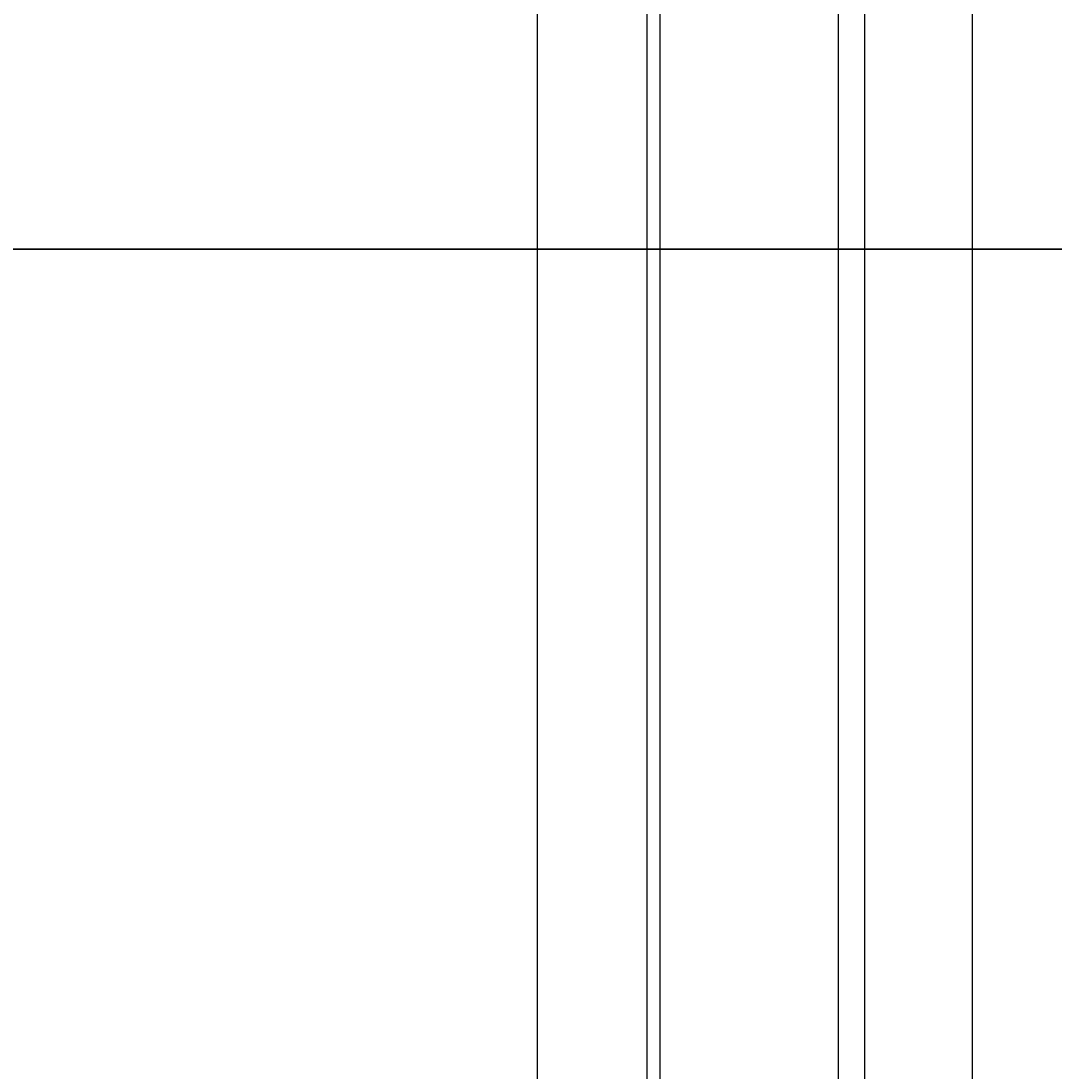
# Model space of a CAD drawing. Units: inches. Extents: x -6 to 289, y -8 to 323.
# Tile 81 of 107: x 150 to 173, y 229 to 252. Entities that reach past the tile are written whole.
import ezdxf

# ---------------------------------------------------------------- set-up
doc = ezdxf.new("R2010")
doc.units = ezdxf.units.IN
doc.header["$MEASUREMENT"] = 0
doc.layers.add('A-ANNO-DIMS', color=2, linetype='Continuous', lineweight=18)
doc.layers.add('A-ELEV', color=7, linetype='Continuous', lineweight=35)
doc.styles.get("Standard").update_dxf_attribs({"font": 'arial.ttf'})
doc.dimstyles.get("Standard").update_dxf_attribs({"dimtxt": 0.18, "dimasz": 0.18, "dimexe": 0.18, "dimexo": 0.0625, "dimgap": 0.09, "dimtad": 0, "dimtih": 1, "dimtoh": 1, "dimdec": 4, "dimzin": 0, "dimdsep": 46, "dimtxsty": 'Standard', "dimcen": 0.09, "dimadec": 0, "dimazin": 0, "dimtfac": 1, "dimtdec": 4, "dimtofl": 0, "dimtmove": 0, "dimatfit": 3, "dimfxl": 1, "dimtolj": 1, "dimtzin": 0, "dimarcsym": 0})

# ---------------------------------------------------------------- blocks, each defined once
blk = doc.blocks.new('*D11')
at = {"layer": 'A-ANNO-DIMS', "color": 0, "lineweight": -2, "transparency": 16777216}
for p, q in [((126.883, 226.717), (126.883, 322.969)), ((168.883, 226.717), (168.883, 322.969)), ((127.063, 322.789), (147.662, 322.789)), ((168.703, 322.789), (148.105, 322.789))]:
    blk.add_line(p, q, dxfattribs=at)
at = {"layer": 'A-ANNO-DIMS', "color": 0, "transparency": 16777216}
for points in [[(127.063, 322.819), (127.063, 322.759), (126.883, 322.789)], [(168.703, 322.819), (168.703, 322.759), (168.883, 322.789)]]:
    blk.add_solid(points, dxfattribs=at)
at = {"layer": 'Defpoints', "color": 0, "transparency": 16777216}
for p in [(168.883, 322.789), (126.883, 226.654), (168.883, 226.654)]:
    blk.add_point(p, dxfattribs=at)
at = {"layer": 'A-ANNO-DIMS', "color": 0, "transparency": 16777216, "insert": (147.883, 322.789), "char_height": 0.18, "attachment_point": 5}
blk.add_mtext('\\A1;42', dxfattribs=at)
blk = doc.blocks.new('*D12')
at = {"layer": 'A-ANNO-DIMS', "color": 0, "lineweight": -2, "transparency": 16777216}
for p, q in [((168.883, 226.717), (168.883, 322.969)), ((188.292, 226.951), (188.292, 322.969)), ((169.063, 322.789), (178.22, 322.789)), ((188.112, 322.789), (178.955, 322.789))]:
    blk.add_line(p, q, dxfattribs=at)
at = {"layer": 'A-ANNO-DIMS', "color": 0, "transparency": 16777216}
for points in [[(169.063, 322.819), (169.063, 322.759), (168.883, 322.789)], [(188.112, 322.819), (188.112, 322.759), (188.292, 322.789)]]:
    blk.add_solid(points, dxfattribs=at)
at = {"layer": 'Defpoints', "color": 0, "transparency": 16777216}
for p in [(188.292, 322.789), (188.292, 226.889), (168.883, 226.654)]:
    blk.add_point(p, dxfattribs=at)
at = {"layer": 'A-ANNO-DIMS', "color": 0, "transparency": 16777216, "insert": (178.588, 322.789), "char_height": 0.18, "attachment_point": 5}
blk.add_mtext('\\A1;19.41', dxfattribs=at)
blk = doc.blocks.new('*D26')
at = {"layer": 'A-ANNO-DIMS', "color": 0, "lineweight": -2, "transparency": 16777216}
for p, q in [((247.226, 247.289), (288.653, 247.289)), ((288.473, 247.109), (288.473, 237.153)), ((288.473, 226.834), (288.473, 236.789)), ((126.946, 226.654), (288.653, 226.654))]:
    blk.add_line(p, q, dxfattribs=at)
at = {"layer": 'A-ANNO-DIMS', "color": 0, "transparency": 16777216}
for points in [[(288.443, 247.109), (288.503, 247.109), (288.473, 247.289)], [(288.443, 226.834), (288.503, 226.834), (288.473, 226.654)]]:
    blk.add_solid(points, dxfattribs=at)
at = {"layer": 'Defpoints', "color": 0, "transparency": 16777216}
for p in [(247.164, 247.289), (288.473, 247.289), (126.883, 226.654)]:
    blk.add_point(p, dxfattribs=at)
at = {"layer": 'A-ANNO-DIMS', "color": 0, "transparency": 16777216, "insert": (288.473, 236.971), "char_height": 0.18, "attachment_point": 5}
blk.add_mtext('\\A1;20.635', dxfattribs=at)
blk = doc.blocks.new('*D27')
at = {"layer": 'A-ANNO-DIMS', "color": 0, "lineweight": -2, "transparency": 16777216}
for p, q in [((19.226, 307.289), (288.653, 307.289)), ((288.473, 307.109), (288.473, 277.471)), ((288.473, 247.469), (288.473, 277.107)), ((247.226, 247.289), (288.653, 247.289))]:
    blk.add_line(p, q, dxfattribs=at)
at = {"layer": 'A-ANNO-DIMS', "color": 0, "transparency": 16777216}
for points in [[(288.443, 307.109), (288.503, 307.109), (288.473, 307.289)], [(288.443, 247.469), (288.503, 247.469), (288.473, 247.289)]]:
    blk.add_solid(points, dxfattribs=at)
at = {"layer": 'Defpoints', "color": 0, "transparency": 16777216}
for p in [(19.164, 307.289), (288.473, 307.289), (247.164, 247.289)]:
    blk.add_point(p, dxfattribs=at)
at = {"layer": 'A-ANNO-DIMS', "color": 0, "transparency": 16777216, "insert": (288.473, 277.289), "char_height": 0.18, "attachment_point": 5}
blk.add_mtext('\\A1;60', dxfattribs=at)
blk = doc.blocks.new('*D76')
at = {"layer": 'A-ANNO-DIMS', "color": 0, "lineweight": -2, "transparency": 16777216}
for p, q in [((142.296, 51.148), (142.296, 322.969)), ((164.296, 51.148), (164.296, 322.969)), ((142.476, 322.789), (153.076, 322.789)), ((164.116, 322.789), (153.516, 322.789))]:
    blk.add_line(p, q, dxfattribs=at)
at = {"layer": 'A-ANNO-DIMS', "color": 0, "transparency": 16777216}
for points in [[(142.476, 322.819), (142.476, 322.759), (142.296, 322.789)], [(164.116, 322.819), (164.116, 322.759), (164.296, 322.789)]]:
    blk.add_solid(points, dxfattribs=at)
at = {"layer": 'Defpoints', "color": 0, "transparency": 16777216}
for p in [(164.296, 322.789), (142.296, 51.085), (164.296, 51.085)]:
    blk.add_point(p, dxfattribs=at)
at = {"layer": 'A-ANNO-DIMS', "color": 0, "transparency": 16777216, "insert": (153.296, 322.789), "char_height": 0.18, "attachment_point": 5}
blk.add_mtext('\\A1;22', dxfattribs=at)
blk = doc.blocks.new('*D77')
at = {"layer": 'A-ANNO-DIMS', "color": 0, "lineweight": -2, "transparency": 16777216}
for p, q in [((164.296, 51.148), (164.296, 322.969)), ((168.296, 51.148), (168.296, 322.969)), ((164.476, 322.789), (166.144, 322.789)), ((168.116, 322.789), (166.448, 322.789))]:
    blk.add_line(p, q, dxfattribs=at)
at = {"layer": 'A-ANNO-DIMS', "color": 0, "transparency": 16777216}
for points in [[(164.476, 322.819), (164.476, 322.759), (164.296, 322.789)], [(168.116, 322.819), (168.116, 322.759), (168.296, 322.789)]]:
    blk.add_solid(points, dxfattribs=at)
at = {"layer": 'Defpoints', "color": 0, "transparency": 16777216}
for p in [(168.296, 322.789), (164.296, 51.085), (168.296, 51.085)]:
    blk.add_point(p, dxfattribs=at)
at = {"layer": 'A-ANNO-DIMS', "color": 0, "transparency": 16777216, "insert": (166.296, 322.789), "char_height": 0.18, "attachment_point": 5}
blk.add_mtext('\\A1;4', dxfattribs=at)
blk = doc.blocks.new('*D78')
at = {"layer": 'A-ANNO-DIMS', "color": 0, "lineweight": -2, "transparency": 16777216}
for p, q in [((168.296, 51.148), (168.296, 322.969)), ((171.296, 51.148), (171.296, 322.969)), ((168.476, 322.789), (169.647, 322.789)), ((171.116, 322.789), (169.945, 322.789))]:
    blk.add_line(p, q, dxfattribs=at)
at = {"layer": 'A-ANNO-DIMS', "color": 0, "transparency": 16777216}
for points in [[(168.476, 322.819), (168.476, 322.759), (168.296, 322.789)], [(171.116, 322.819), (171.116, 322.759), (171.296, 322.789)]]:
    blk.add_solid(points, dxfattribs=at)
at = {"layer": 'Defpoints', "color": 0, "transparency": 16777216}
for p in [(171.296, 322.789), (168.296, 51.085), (171.296, 51.085)]:
    blk.add_point(p, dxfattribs=at)
at = {"layer": 'A-ANNO-DIMS', "color": 0, "transparency": 16777216, "insert": (169.796, 322.789), "char_height": 0.18, "attachment_point": 5}
blk.add_mtext('\\A1;3', dxfattribs=at)
blk = doc.blocks.new('*D79')
at = {"layer": 'A-ANNO-DIMS', "color": 0, "lineweight": -2, "transparency": 16777216}
for p, q in [((171.296, 118.033), (171.296, 322.969)), ((188.292, 116.842), (188.292, 322.969)), ((171.476, 322.789), (179.339, 322.789)), ((188.112, 322.789), (180.249, 322.789))]:
    blk.add_line(p, q, dxfattribs=at)
at = {"layer": 'A-ANNO-DIMS', "color": 0, "transparency": 16777216}
for points in [[(171.476, 322.819), (171.476, 322.759), (171.296, 322.789)], [(188.112, 322.819), (188.112, 322.759), (188.292, 322.789)]]:
    blk.add_solid(points, dxfattribs=at)
at = {"layer": 'Defpoints', "color": 0, "transparency": 16777216}
for p in [(188.292, 322.789), (171.296, 117.971), (188.292, 116.779)]:
    blk.add_point(p, dxfattribs=at)
at = {"layer": 'A-ANNO-DIMS', "color": 0, "transparency": 16777216, "insert": (179.794, 322.789), "char_height": 0.18, "attachment_point": 5}
blk.add_mtext('\\A1;16.996', dxfattribs=at)
blk = doc.blocks.new('*D94')
at = {"layer": 'A-ANNO-DIMS', "color": 0, "lineweight": -2, "transparency": 16777216}
for p, q in [((118.164, 159.411), (118.164, 322.969)), ((161.552, 159.411), (161.552, 322.969)), ((118.344, 322.789), (139.46, 322.789)), ((161.372, 322.789), (140.256, 322.789))]:
    blk.add_line(p, q, dxfattribs=at)
at = {"layer": 'A-ANNO-DIMS', "color": 0, "transparency": 16777216}
for points in [[(118.344, 322.819), (118.344, 322.759), (118.164, 322.789)], [(161.372, 322.819), (161.372, 322.759), (161.552, 322.789)]]:
    blk.add_solid(points, dxfattribs=at)
at = {"layer": 'Defpoints', "color": 0, "transparency": 16777216}
for p in [(161.552, 322.789), (118.164, 159.348), (161.552, 159.348)]:
    blk.add_point(p, dxfattribs=at)
at = {"layer": 'A-ANNO-DIMS', "color": 0, "transparency": 16777216, "insert": (139.858, 322.789), "char_height": 0.18, "attachment_point": 5}
blk.add_mtext('\\A1;43.39', dxfattribs=at)
blk = doc.blocks.new('*D95')
at = {"layer": 'A-ANNO-DIMS', "color": 0, "lineweight": -2, "transparency": 16777216}
for p, q in [((161.552, 159.411), (161.552, 322.969)), ((164.004, 159.411), (164.004, 322.969)), ((161.732, 322.789), (162.452, 322.789)), ((163.824, 322.789), (163.104, 322.789))]:
    blk.add_line(p, q, dxfattribs=at)
at = {"layer": 'A-ANNO-DIMS', "color": 0, "transparency": 16777216}
for points in [[(161.732, 322.819), (161.732, 322.759), (161.552, 322.789)], [(163.824, 322.819), (163.824, 322.759), (164.004, 322.789)]]:
    blk.add_solid(points, dxfattribs=at)
at = {"layer": 'Defpoints', "color": 0, "transparency": 16777216}
for p in [(164.004, 322.789), (161.552, 159.348), (164.004, 159.348)]:
    blk.add_point(p, dxfattribs=at)
at = {"layer": 'A-ANNO-DIMS', "color": 0, "transparency": 16777216, "insert": (162.778, 322.789), "char_height": 0.18, "attachment_point": 5}
blk.add_mtext('\\A1;2.45', dxfattribs=at)
blk = doc.blocks.new('*D96')
at = {"layer": 'A-ANNO-DIMS', "color": 0, "lineweight": -2, "transparency": 16777216}
for p, q in [((164.004, 159.411), (164.004, 322.969)), ((200.616, 159.411), (200.616, 322.969)), ((164.184, 322.789), (181.934, 322.789)), ((200.436, 322.789), (182.686, 322.789))]:
    blk.add_line(p, q, dxfattribs=at)
at = {"layer": 'A-ANNO-DIMS', "color": 0, "transparency": 16777216}
for points in [[(164.184, 322.819), (164.184, 322.759), (164.004, 322.789)], [(200.436, 322.819), (200.436, 322.759), (200.616, 322.789)]]:
    blk.add_solid(points, dxfattribs=at)
at = {"layer": 'Defpoints', "color": 0, "transparency": 16777216}
for p in [(200.616, 322.789), (164.004, 159.348), (200.616, 159.348)]:
    blk.add_point(p, dxfattribs=at)
at = {"layer": 'A-ANNO-DIMS', "color": 0, "transparency": 16777216, "insert": (182.31, 322.789), "char_height": 0.18, "attachment_point": 5}
blk.add_mtext('\\A1;36.61', dxfattribs=at)

msp = doc.modelspace()

# ---------------------------------------------------------------- linework, layer by layer
at = {"layer": 'A-ELEV'}
for p, q in [((247.1638, 247.2888), (115.1638, 247.2888)), ((115.1638, 247.2888), (247.1638, 247.2888))]:
    msp.add_line(p, q, dxfattribs=at)

# ---------------------------------------------------------------- dimensions: what is measured, and where the dimension line sits
at = {"layer": 'A-ANNO-DIMS'}
for base, p1, p2, override, picture, middle in [((161.5522, 322.7888), (118.1638, 159.3484), (161.5522, 159.3484), {"dimdec": 2, "dimlfac": 1, "dimrnd": 0, "dimzin": 0, "dimdsep": 46, "dimlunit": 2}, '*D94', (139.858, 322.7888)), ((168.8835, 322.7888), (126.8835, 226.654), (168.8835, 226.654), {"dimdec": 0, "dimlfac": 1, "dimrnd": 0, "dimzin": 0, "dimdsep": 46, "dimlunit": 2}, '*D11', (147.8835, 322.7888)), ((164.296, 322.7888), (142.296, 51.0851), (164.296, 51.0851), {"dimdec": 0, "dimlfac": 1, "dimrnd": 0, "dimzin": 0, "dimdsep": 46, "dimlunit": 2}, '*D76', (153.296, 322.7888)), ((164.0039, 322.7888), (161.5522, 159.3484), (164.0039, 159.3484), {"dimdec": 2, "dimlfac": 1, "dimrnd": 0, "dimzin": 0, "dimdsep": 46, "dimlunit": 2}, '*D95', (162.7781, 322.7888)), ((200.6162, 322.7888), (164.0039, 159.3484), (200.6162, 159.3484), {"dimdec": 2, "dimlfac": 1, "dimrnd": 0, "dimzin": 0, "dimdsep": 46, "dimlunit": 2}, '*D96', (182.3101, 322.7888)), ((168.296, 322.7888), (164.296, 51.0851), (168.296, 51.0851), {"dimdec": 0, "dimlfac": 1, "dimrnd": 0, "dimzin": 0, "dimdsep": 46, "dimlunit": 2}, '*D77', (166.296, 322.7888)), ((171.296, 322.7888), (168.296, 51.0851), (171.296, 51.0851), {"dimdec": 0, "dimlfac": 1, "dimrnd": 0, "dimzin": 0, "dimdsep": 46, "dimlunit": 2}, '*D78', (169.796, 322.7888)), ((188.2918, 322.7888), (168.8835, 226.654), (188.2918, 226.8887), {"dimdec": 2, "dimlfac": 1, "dimrnd": 0, "dimzin": 0, "dimdsep": 46, "dimlunit": 2}, '*D12', (178.5876, 322.7888)), ((188.2918, 322.7888), (171.296, 117.9706), (188.2918, 116.7795), {"dimdec": 3, "dimlfac": 1, "dimrnd": 0, "dimzin": 0, "dimdsep": 46, "dimlunit": 2}, '*D79', (179.7939, 322.7888))]:
    dim = msp.add_linear_dim(base=base, p1=p1, p2=p2, dimstyle='Standard', override=override, dxfattribs=at)
    dim.commit()
    dim.dimension.update_dxf_attribs({"geometry": picture, "text_midpoint": middle})
for base, p1, p2, override, picture, middle in [((288.4733, 307.2888), (247.1638, 247.2888), (19.1638, 307.2888), {"dimdec": 0, "dimlfac": 1, "dimrnd": 0, "dimzin": 0, "dimdsep": 46, "dimlunit": 2}, '*D27', (288.4733, 277.2888)), ((288.4733, 247.2888), (126.8835, 226.654), (247.1638, 247.2888), {"dimdec": 3, "dimlfac": 1, "dimrnd": 0, "dimzin": 0, "dimdsep": 46, "dimlunit": 2}, '*D26', (288.4733, 236.9714))]:
    dim = msp.add_linear_dim(base=base, p1=p1, p2=p2, angle=90, dimstyle='Standard', override=override, dxfattribs=at)
    dim.commit()
    dim.dimension.update_dxf_attribs({"geometry": picture, "text_midpoint": middle})

doc.saveas('drawing.dxf')
